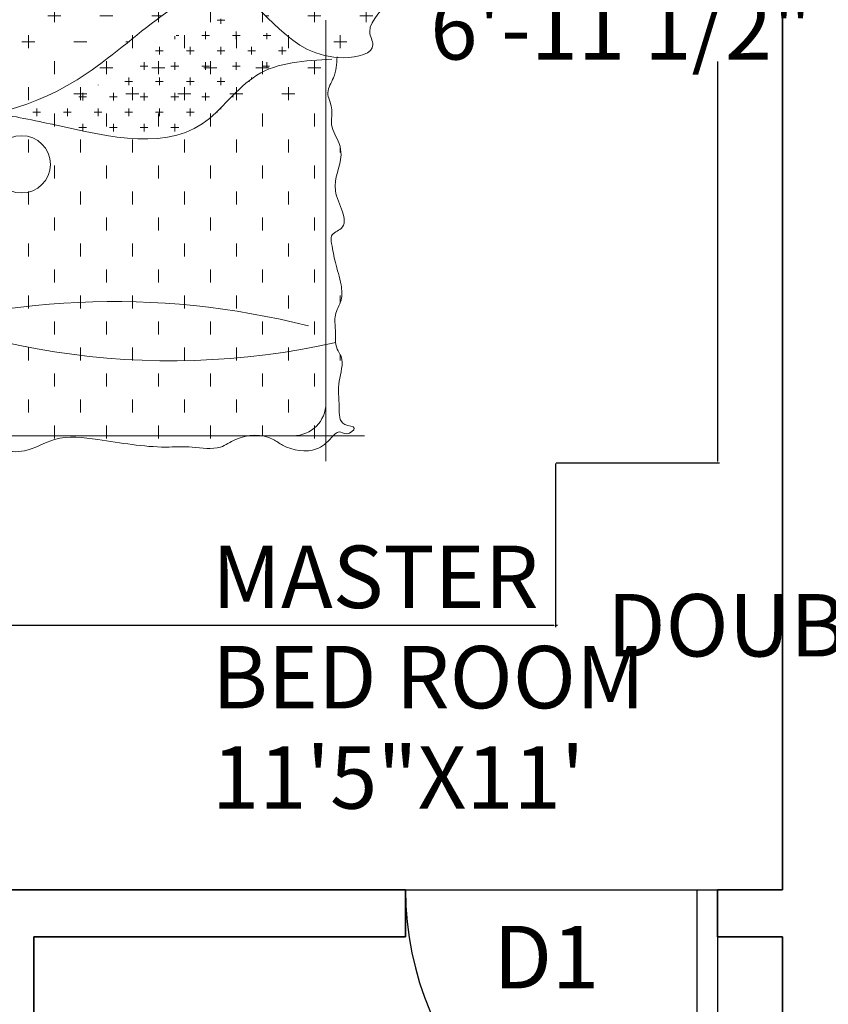
# Model space of a CAD drawing. Units: inches. Extents: x -26 to 575, y -18 to 513.
# Tile 12 of 28: x 196 to 274, y 324 to 418. Entities that reach past the tile are written whole.
import ezdxf

# ---------------------------------------------------------------- set-up
doc = ezdxf.new("R2010")
doc.units = ezdxf.units.IN
doc.header["$MEASUREMENT"] = 0
for name, color, linetype, lineweight in [('A-ANNO-DIMS', 2, 'Continuous', 18), ('A-ANNO-TEXT', 7, 'Continuous', 18), ('A-AREA-IDEN', 7, 'Continuous', 18), ('A-DOOR', 3, 'Continuous', 25), ('A-WALL', 7, 'Continuous', 35), ('Furniture', 8, 'Continuous', 15)]:
    doc.layers.add(name, color=color, linetype=linetype, lineweight=lineweight)
doc.styles.get("Standard").update_dxf_attribs({"font": 'arial.ttf', "height": 6})
doc.dimstyles.get("Standard").update_dxf_attribs({"dimtxt": 6, "dimasz": 0.18, "dimexe": 0.18, "dimexo": 0.0625, "dimgap": 0.09, "dimtad": 0, "dimtih": 1, "dimtoh": 1, "dimzin": 0, "dimdsep": 46, "dimlunit": 3, "dimtxsty": 'Standard', "dimcen": 0.09, "dimadec": 0, "dimazin": 0, "dimtfac": 1, "dimtofl": 0, "dimtmove": 0, "dimatfit": 3, "dimfxl": 1, "dimtolj": 1, "dimtzin": 0, "dimarcsym": 0})

# ---------------------------------------------------------------- blocks, each defined once
blk = doc.blocks.new('BED-DOUBLE-WITH-NIGHTSTANDS')
for p, q in [((1.925, 83.361), (1.925, 62.761)), ((82.669, 83.361), (82.669, 62.761)), ((21.61, 63.031), (21.61, 82.461)), ((22.828, 60.828), (22.828, 82.615)), ((81.883, 82.344), (81.883, 56.232)), ((102.354, 63.031), (102.354, 82.461)), ((10.269, 81.761), (8.938, 70.826)), ((23.226, 81.078), (0, 81.078)), ((21.24, 81.17), (81.883, 81.17)), ((103.97, 81.078), (80.744, 81.078)), ((20.889, 80.153), (2.667, 80.153)), ((2.667, 80.153), (2.667, 64.968)), ((20.889, 64.968), (20.889, 80.153)), ((82.669, 79.717), (21.062, 79.717)), ((101.633, 80.153), (83.411, 80.153)), ((83.411, 80.153), (83.411, 64.968)), ((101.633, 64.968), (101.633, 80.153)), ((92.567, 79.403), (92.567, 67.508)), ((14.667, 76.005), (4.51, 77.257)), ((25.057, 76.764), (22.828, 76.764)), ((41.168, 76.507), (40.96, 76.715)), ((41.168, 76.507), (41.434, 76.772)), ((41.169, 76.507), (41.169, 76.741)), ((56.226, 76.764), (41.357, 76.764)), ((43.997, 76.507), (43.732, 76.772)), ((43.997, 76.507), (43.997, 76.882)), ((43.997, 76.507), (44.262, 76.772)), ((46.825, 76.507), (46.56, 76.772)), ((46.825, 76.507), (47.09, 76.772)), ((46.826, 76.507), (46.826, 76.882)), ((57.003, 76.507), (56.737, 76.772)), ((57.003, 76.507), (57.003, 76.828)), ((57.003, 76.507), (57.268, 76.772)), ((81.883, 76.764), (59.394, 76.764)), ((59.831, 76.507), (59.594, 76.744)), ((59.831, 76.507), (59.831, 76.717)), ((59.831, 76.507), (60.018, 76.694)), ((8.056, 67.244), (12.026, 75.725)), ((12.026, 75.725), (14.235, 74.691)), ((11.458, 75.323), (8.122, 68.196)), ((11.769, 75.177), (11.458, 75.323)), ((25.612, 75.093), (25.347, 75.358)), ((25.612, 75.093), (25.612, 75.468)), ((25.612, 75.093), (25.877, 75.358)), ((28.44, 75.093), (28.175, 75.358)), ((28.44, 75.093), (28.706, 75.358)), ((28.441, 75.093), (28.441, 75.468)), ((31.269, 75.093), (31.004, 75.358)), ((31.269, 75.093), (31.269, 75.468)), ((31.269, 75.093), (31.534, 75.358)), ((34.097, 75.093), (33.832, 75.358)), ((34.097, 75.093), (34.362, 75.358)), ((34.098, 75.093), (34.098, 75.468)), ((36.926, 75.093), (36.661, 75.358)), ((36.926, 75.093), (36.926, 75.468)), ((36.926, 75.093), (37.191, 75.358)), ((39.754, 75.093), (39.489, 75.358)), ((39.754, 75.093), (40.019, 75.358)), ((39.755, 75.093), (39.755, 75.468)), ((42.583, 75.093), (42.317, 75.358)), ((42.583, 75.093), (42.583, 75.468)), ((42.583, 75.093), (42.848, 75.358)), ((45.411, 75.093), (45.146, 75.358)), ((45.411, 75.093), (45.411, 75.468)), ((45.411, 75.093), (45.676, 75.358)), ((48.239, 75.093), (47.974, 75.358)), ((48.239, 75.093), (48.505, 75.358)), ((48.24, 75.093), (48.24, 75.468)), ((51.068, 75.093), (50.803, 75.358)), ((51.068, 75.093), (51.068, 75.099)), ((51.068, 75.093), (51.07, 75.095)), ((53.004, 75.337), (53.025, 75.358)), ((55.588, 75.093), (55.323, 75.358)), ((55.588, 75.093), (55.854, 75.358)), ((55.589, 75.093), (55.589, 75.468)), ((58.417, 75.093), (58.152, 75.358)), ((58.417, 75.093), (58.417, 75.468)), ((58.417, 75.093), (58.682, 75.358)), ((61.245, 75.093), (60.98, 75.358)), ((61.245, 75.093), (61.51, 75.358)), ((61.246, 75.093), (61.246, 75.468)), ((64.074, 75.093), (63.809, 75.358)), ((64.074, 75.093), (64.074, 75.468)), ((64.074, 75.093), (64.339, 75.358)), ((66.902, 75.093), (66.637, 75.358)), ((66.902, 75.093), (67.167, 75.358)), ((66.903, 75.093), (66.903, 75.468)), ((69.731, 75.093), (69.465, 75.358)), ((69.731, 75.093), (69.731, 75.468)), ((69.731, 75.093), (69.996, 75.358)), ((72.559, 75.093), (72.294, 75.358)), ((72.559, 75.093), (72.559, 75.468)), ((72.559, 75.093), (72.824, 75.358)), ((75.387, 75.093), (75.122, 75.358)), ((75.387, 75.093), (75.653, 75.358)), ((75.388, 75.093), (75.388, 75.468)), ((78.216, 75.093), (77.951, 75.358)), ((78.216, 75.093), (78.216, 75.468)), ((78.216, 75.093), (78.481, 75.358)), ((14.235, 74.691), (10.265, 66.21)), ((19.14, 71.727), (13.978, 74.143)), ((27.026, 73.679), (26.761, 73.944)), ((27.026, 73.679), (27.291, 73.944)), ((27.027, 73.678), (27.027, 74.053)), ((29.855, 73.679), (29.589, 73.944)), ((29.855, 73.678), (29.855, 74.053)), ((29.855, 73.679), (30.12, 73.944)), ((32.683, 73.679), (32.418, 73.944)), ((32.683, 73.678), (32.683, 74.053)), ((32.683, 73.679), (32.948, 73.944)), ((35.512, 73.679), (35.246, 73.944)), ((35.512, 73.678), (35.512, 74.053)), ((35.512, 73.679), (35.777, 73.944)), ((38.34, 73.679), (38.075, 73.944)), ((38.34, 73.678), (38.34, 74.053)), ((38.34, 73.679), (38.605, 73.944)), ((41.168, 73.679), (40.903, 73.944)), ((41.168, 73.679), (41.434, 73.944)), ((41.169, 73.678), (41.169, 74.053)), ((43.997, 73.679), (43.732, 73.944)), ((43.997, 73.678), (43.997, 74.053)), ((43.997, 73.679), (44.262, 73.944)), ((46.825, 73.679), (46.56, 73.944)), ((46.825, 73.679), (47.09, 73.944)), ((46.826, 73.678), (46.826, 74.053)), ((49.654, 73.679), (49.388, 73.944)), ((49.654, 73.678), (49.654, 74.053)), ((49.654, 73.679), (49.919, 73.944)), ((54.174, 73.679), (53.909, 73.944)), ((54.174, 73.679), (54.439, 73.944)), ((54.175, 73.678), (54.175, 74.053)), ((57.003, 73.679), (56.737, 73.944)), ((57.003, 73.678), (57.003, 74.053)), ((57.003, 73.679), (57.268, 73.944)), ((59.831, 73.679), (59.566, 73.944)), ((59.831, 73.678), (59.831, 74.053)), ((59.831, 73.679), (60.096, 73.944)), ((62.66, 73.679), (62.394, 73.944)), ((62.66, 73.678), (62.66, 74.053)), ((62.66, 73.679), (62.925, 73.944)), ((65.488, 73.679), (65.223, 73.944)), ((65.488, 73.678), (65.488, 74.053)), ((65.488, 73.679), (65.753, 73.944)), ((68.316, 73.679), (68.051, 73.944)), ((68.316, 73.679), (68.582, 73.944)), ((68.317, 73.678), (68.317, 74.053)), ((71.145, 73.679), (70.88, 73.944)), ((71.145, 73.678), (71.145, 74.053)), ((71.145, 73.679), (71.41, 73.944)), ((73.973, 73.679), (73.708, 73.944)), ((73.973, 73.679), (74.238, 73.944)), ((73.974, 73.678), (73.974, 74.053)), ((76.802, 73.679), (76.536, 73.944)), ((76.802, 73.678), (76.802, 74.053)), ((76.802, 73.679), (77.067, 73.944)), ((79.63, 73.679), (79.365, 73.944)), ((79.63, 73.678), (79.63, 74.053)), ((79.63, 73.679), (79.895, 73.944)), ((13.242, 72.571), (11.033, 73.605)), ((14.129, 73), (11.598, 67.591)), ((17.984, 71.195), (14.129, 73)), ((98.466, 73.144), (86.668, 73.144)), ((25.612, 72.265), (25.347, 72.53)), ((25.612, 72.264), (25.612, 72.639)), ((25.612, 72.265), (25.877, 72.53)), ((28.44, 72.265), (28.175, 72.53)), ((28.44, 72.265), (28.706, 72.53)), ((28.441, 72.264), (28.441, 72.639)), ((31.269, 72.265), (31.004, 72.53)), ((31.269, 72.264), (31.269, 72.639)), ((31.269, 72.265), (31.534, 72.53)), ((34.097, 72.265), (33.832, 72.53)), ((34.097, 72.265), (34.362, 72.53)), ((34.098, 72.264), (34.098, 72.639)), ((36.926, 72.265), (36.661, 72.53)), ((36.926, 72.264), (36.926, 72.639)), ((36.926, 72.265), (37.191, 72.53)), ((39.754, 72.265), (39.489, 72.53)), ((39.754, 72.265), (40.019, 72.53)), ((39.755, 72.264), (39.755, 72.639)), ((42.583, 72.265), (42.317, 72.53)), ((42.583, 72.264), (42.583, 72.639)), ((42.583, 72.265), (42.848, 72.53)), ((45.411, 72.265), (45.146, 72.53)), ((45.411, 72.264), (45.411, 72.639)), ((45.411, 72.265), (45.676, 72.53)), ((48.239, 72.265), (47.974, 72.53)), ((48.239, 72.265), (48.505, 72.53)), ((48.24, 72.264), (48.24, 72.639)), ((55.588, 72.265), (55.323, 72.53)), ((55.588, 72.265), (55.854, 72.53)), ((55.589, 72.264), (55.589, 72.639)), ((58.417, 72.265), (58.152, 72.53)), ((58.417, 72.264), (58.417, 72.639)), ((58.417, 72.265), (58.682, 72.53)), ((61.245, 72.265), (60.98, 72.53)), ((61.245, 72.265), (61.51, 72.53)), ((61.246, 72.264), (61.246, 72.639)), ((64.074, 72.265), (63.809, 72.53)), ((64.074, 72.264), (64.074, 72.639)), ((64.074, 72.265), (64.339, 72.53)), ((66.902, 72.265), (66.637, 72.53)), ((66.902, 72.265), (67.167, 72.53)), ((66.903, 72.264), (66.903, 72.639)), ((69.731, 72.265), (69.465, 72.53)), ((69.731, 72.264), (69.731, 72.639)), ((69.731, 72.265), (69.996, 72.53)), ((72.559, 72.265), (72.294, 72.53)), ((72.559, 72.264), (72.559, 72.639)), ((72.559, 72.265), (72.824, 72.53)), ((75.387, 72.265), (75.122, 72.53)), ((75.387, 72.265), (75.653, 72.53)), ((75.388, 72.264), (75.388, 72.639)), ((78.216, 72.265), (77.951, 72.53)), ((78.216, 72.264), (78.216, 72.639)), ((78.216, 72.265), (78.481, 72.53)), ((15.452, 65.787), (17.984, 71.195)), ((15.804, 64.601), (19.14, 71.727)), ((24.198, 70.85), (23.972, 71.076)), ((24.198, 70.85), (24.198, 71.225)), ((24.198, 70.85), (24.463, 71.116)), ((27.026, 70.85), (26.761, 71.116)), ((27.026, 70.85), (27.291, 71.116)), ((27.027, 70.85), (27.027, 71.225)), ((29.855, 70.85), (29.589, 71.116)), ((29.855, 70.85), (29.855, 71.225)), ((29.855, 70.85), (30.12, 71.116)), ((32.683, 70.85), (32.418, 71.116)), ((32.683, 70.85), (32.683, 71.225)), ((32.683, 70.85), (32.948, 71.116)), ((35.512, 70.85), (35.246, 71.116)), ((35.512, 70.85), (35.512, 71.225)), ((35.512, 70.85), (35.777, 71.116)), ((38.34, 70.85), (38.075, 71.116)), ((38.34, 70.85), (38.34, 71.225)), ((38.34, 70.85), (38.605, 71.116)), ((41.168, 70.85), (40.903, 71.116)), ((41.168, 70.85), (41.434, 71.116)), ((41.169, 70.85), (41.169, 71.225)), ((43.997, 70.85), (43.732, 71.116)), ((43.997, 70.85), (43.997, 71.225)), ((43.997, 70.85), (44.262, 71.116)), ((46.825, 70.85), (46.56, 71.116)), ((46.825, 70.85), (47.09, 71.116)), ((46.826, 70.85), (46.826, 71.225)), ((49.654, 70.85), (49.388, 71.116)), ((49.654, 70.85), (49.654, 71.225)), ((49.654, 70.85), (49.919, 71.116)), ((54.174, 70.85), (53.909, 71.116)), ((54.174, 70.85), (54.439, 71.116)), ((54.175, 70.85), (54.175, 71.225)), ((57.003, 70.85), (56.737, 71.116)), ((57.003, 70.85), (57.003, 71.225)), ((57.003, 70.85), (57.268, 71.116)), ((59.831, 70.85), (59.566, 71.116)), ((59.831, 70.85), (59.831, 71.225)), ((59.831, 70.85), (60.096, 71.116)), ((62.66, 70.85), (62.394, 71.116)), ((62.66, 70.85), (62.66, 71.225)), ((62.66, 70.85), (62.925, 71.116)), ((65.488, 70.85), (65.223, 71.116)), ((65.488, 70.85), (65.488, 71.225)), ((65.488, 70.85), (65.753, 71.116)), ((68.316, 70.85), (68.051, 71.116)), ((68.316, 70.85), (68.582, 71.116)), ((68.317, 70.85), (68.317, 71.225)), ((71.145, 70.85), (70.88, 71.116)), ((71.145, 70.85), (71.145, 71.225)), ((71.145, 70.85), (71.41, 71.116)), ((73.973, 70.85), (73.708, 71.116)), ((73.973, 70.85), (74.238, 71.116)), ((73.974, 70.85), (73.974, 71.225)), ((76.802, 70.85), (76.536, 71.116)), ((76.802, 70.85), (76.802, 71.225)), ((76.802, 70.85), (77.067, 71.116)), ((79.63, 70.85), (79.365, 71.116)), ((79.63, 70.85), (79.63, 71.225)), ((79.63, 70.85), (79.895, 71.116)), ((11.136, 68.071), (8.927, 69.105)), ((25.612, 69.436), (25.347, 69.701)), ((25.612, 69.436), (25.612, 69.811)), ((25.612, 69.436), (25.877, 69.701)), ((28.44, 69.436), (28.175, 69.701)), ((28.44, 69.436), (28.706, 69.701)), ((28.441, 69.436), (28.441, 69.811)), ((31.269, 69.436), (31.004, 69.701)), ((31.269, 69.436), (31.269, 69.811)), ((31.269, 69.436), (31.534, 69.701)), ((34.097, 69.436), (33.832, 69.701)), ((34.097, 69.436), (34.362, 69.701)), ((34.098, 69.436), (34.098, 69.811)), ((36.926, 69.436), (36.661, 69.701)), ((36.926, 69.436), (36.926, 69.811)), ((36.926, 69.436), (37.191, 69.701)), ((39.754, 69.436), (39.489, 69.701)), ((39.754, 69.436), (40.019, 69.701)), ((39.755, 69.436), (39.755, 69.811)), ((42.583, 69.436), (42.317, 69.701)), ((42.583, 69.436), (42.583, 69.811)), ((42.583, 69.436), (42.848, 69.701)), ((45.411, 69.436), (45.146, 69.701)), ((45.411, 69.436), (45.411, 69.811)), ((45.411, 69.436), (45.676, 69.701)), ((48.239, 69.436), (47.974, 69.701)), ((48.239, 69.436), (48.505, 69.701)), ((48.24, 69.436), (48.24, 69.811)), ((51.052, 69.452), (50.803, 69.701)), ((53.007, 69.683), (53.025, 69.701)), ((55.588, 69.436), (55.323, 69.701)), ((55.588, 69.436), (55.854, 69.701)), ((55.589, 69.436), (55.589, 69.811)), ((58.417, 69.436), (58.152, 69.701)), ((58.417, 69.436), (58.417, 69.811)), ((58.417, 69.436), (58.682, 69.701)), ((61.245, 69.436), (60.98, 69.701)), ((61.245, 69.436), (61.51, 69.701)), ((61.246, 69.436), (61.246, 69.811)), ((64.074, 69.436), (63.809, 69.701)), ((64.074, 69.436), (64.074, 69.811)), ((64.074, 69.436), (64.339, 69.701)), ((66.902, 69.436), (66.637, 69.701)), ((66.902, 69.436), (67.167, 69.701)), ((66.903, 69.436), (66.903, 69.811)), ((69.731, 69.436), (69.465, 69.701)), ((69.731, 69.436), (69.731, 69.811)), ((69.731, 69.436), (69.996, 69.701)), ((72.559, 69.436), (72.294, 69.701)), ((72.559, 69.436), (72.559, 69.811)), ((72.559, 69.436), (72.824, 69.701)), ((75.387, 69.436), (75.122, 69.701)), ((75.387, 69.436), (75.653, 69.701)), ((75.388, 69.436), (75.388, 69.811)), ((78.216, 69.436), (77.951, 69.701)), ((78.216, 69.436), (78.216, 69.811)), ((78.216, 69.436), (78.481, 69.701)), ((8.122, 68.196), (8.434, 68.05)), ((24.198, 68.022), (23.933, 68.287)), ((24.198, 68.022), (24.198, 68.397)), ((24.198, 68.022), (24.463, 68.287)), ((27.026, 68.022), (26.761, 68.287)), ((27.026, 68.022), (27.291, 68.287)), ((27.027, 68.022), (27.027, 68.397)), ((29.855, 68.022), (29.589, 68.287)), ((29.855, 68.022), (29.855, 68.397)), ((29.855, 68.022), (30.12, 68.287)), ((32.683, 68.022), (32.418, 68.287)), ((32.683, 68.022), (32.683, 68.397)), ((32.683, 68.022), (32.948, 68.287)), ((35.512, 68.022), (35.246, 68.287)), ((35.512, 68.022), (35.512, 68.397)), ((35.512, 68.022), (35.777, 68.287)), ((38.34, 68.022), (38.075, 68.287)), ((38.34, 68.022), (38.34, 68.397)), ((38.34, 68.022), (38.605, 68.287)), ((41.168, 68.022), (40.903, 68.287)), ((41.168, 68.022), (41.434, 68.287)), ((41.169, 68.022), (41.169, 68.397)), ((43.997, 68.022), (43.732, 68.287)), ((43.997, 68.022), (43.997, 68.397)), ((43.997, 68.022), (44.262, 68.287)), ((46.825, 68.022), (46.56, 68.287)), ((46.825, 68.022), (47.09, 68.287)), ((46.826, 68.022), (46.826, 68.397)), ((49.654, 68.022), (49.388, 68.287)), ((49.654, 68.022), (49.654, 68.397)), ((49.654, 68.022), (49.919, 68.287)), ((54.174, 68.022), (53.909, 68.287)), ((54.174, 68.022), (54.439, 68.287)), ((54.175, 68.022), (54.175, 68.397)), ((57.003, 68.022), (56.737, 68.287)), ((57.003, 68.022), (57.003, 68.397)), ((57.003, 68.022), (57.268, 68.287)), ((59.831, 68.022), (59.566, 68.287)), ((59.831, 68.022), (59.831, 68.397)), ((59.831, 68.022), (60.096, 68.287)), ((62.66, 68.022), (62.394, 68.287)), ((62.66, 68.022), (62.66, 68.397)), ((62.66, 68.022), (62.925, 68.287)), ((65.488, 68.022), (65.223, 68.287)), ((65.488, 68.022), (65.488, 68.397)), ((65.488, 68.022), (65.753, 68.287)), ((68.316, 68.022), (68.051, 68.287)), ((68.316, 68.022), (68.582, 68.287)), ((68.317, 68.022), (68.317, 68.397)), ((71.145, 68.022), (70.88, 68.287)), ((71.145, 68.022), (71.145, 68.397)), ((71.145, 68.022), (71.41, 68.287)), ((73.973, 68.022), (73.708, 68.287)), ((73.973, 68.022), (74.238, 68.287)), ((73.974, 68.022), (73.974, 68.397)), ((76.802, 68.022), (76.536, 68.287)), ((76.802, 68.022), (76.802, 68.397)), ((76.802, 68.022), (77.067, 68.287)), ((79.63, 68.022), (79.365, 68.287)), ((79.63, 68.022), (79.63, 68.397)), ((79.63, 68.022), (79.895, 68.287)), ((10.265, 66.21), (8.056, 67.244)), ((11.598, 67.591), (15.452, 65.787)), ((10.642, 67.017), (15.804, 64.601)), ((25.612, 66.608), (25.347, 66.873)), ((25.612, 66.607), (25.612, 66.982)), ((25.612, 66.608), (25.877, 66.873)), ((28.44, 66.608), (28.175, 66.873)), ((28.44, 66.608), (28.706, 66.873)), ((28.441, 66.607), (28.441, 66.982)), ((31.269, 66.608), (31.004, 66.873)), ((31.269, 66.607), (31.269, 66.982)), ((31.269, 66.608), (31.534, 66.873)), ((34.097, 66.608), (33.832, 66.873)), ((34.097, 66.608), (34.362, 66.873)), ((34.098, 66.607), (34.098, 66.982)), ((36.926, 66.608), (36.661, 66.873)), ((36.926, 66.607), (36.926, 66.982)), ((36.926, 66.608), (37.191, 66.873)), ((39.754, 66.608), (39.489, 66.873)), ((39.754, 66.608), (40.019, 66.873)), ((39.755, 66.607), (39.755, 66.982)), ((42.583, 66.608), (42.317, 66.873)), ((42.583, 66.607), (42.583, 66.982)), ((42.583, 66.608), (42.848, 66.873)), ((45.411, 66.608), (45.146, 66.873)), ((45.411, 66.607), (45.411, 66.982)), ((45.411, 66.608), (45.676, 66.873)), ((48.239, 66.608), (47.974, 66.873)), ((48.239, 66.608), (48.505, 66.873)), ((48.24, 66.607), (48.24, 66.982)), ((51.068, 66.608), (50.803, 66.873)), ((51.068, 66.607), (51.068, 66.982)), ((51.068, 66.608), (51.333, 66.873)), ((52.76, 66.608), (52.495, 66.873)), ((52.76, 66.607), (52.76, 66.982)), ((52.76, 66.608), (53.025, 66.873)), ((55.588, 66.608), (55.323, 66.873)), ((55.588, 66.608), (55.854, 66.873)), ((55.589, 66.607), (55.589, 66.982)), ((58.417, 66.608), (58.152, 66.873)), ((58.417, 66.607), (58.417, 66.982)), ((58.417, 66.608), (58.682, 66.873)), ((61.245, 66.608), (60.98, 66.873)), ((61.245, 66.608), (61.51, 66.873)), ((61.246, 66.607), (61.246, 66.982)), ((64.074, 66.608), (63.809, 66.873)), ((64.074, 66.607), (64.074, 66.982)), ((64.074, 66.608), (64.339, 66.873)), ((66.902, 66.608), (66.637, 66.873)), ((66.902, 66.608), (67.167, 66.873)), ((66.903, 66.607), (66.903, 66.982)), ((69.731, 66.608), (69.465, 66.873)), ((69.731, 66.607), (69.731, 66.982)), ((69.731, 66.608), (69.996, 66.873)), ((72.559, 66.608), (72.294, 66.873)), ((72.559, 66.607), (72.559, 66.982)), ((72.559, 66.608), (72.824, 66.873)), ((75.387, 66.608), (75.122, 66.873)), ((75.387, 66.608), (75.653, 66.873)), ((75.388, 66.607), (75.388, 66.982)), ((78.216, 66.608), (77.951, 66.873)), ((78.216, 66.607), (78.216, 66.982)), ((78.216, 66.608), (78.481, 66.873)), ((81.044, 66.608), (80.779, 66.873)), ((81.044, 66.608), (81.253, 66.817)), ((81.045, 66.607), (81.045, 66.982)), ((24.198, 65.385), (24.198, 65.568)), ((24.295, 65.291), (24.463, 65.459)), ((27.026, 65.194), (26.761, 65.459)), ((27.026, 65.194), (27.291, 65.459)), ((27.027, 65.193), (27.027, 65.568)), ((29.855, 65.194), (29.589, 65.459)), ((29.855, 65.193), (29.855, 65.568)), ((29.855, 65.194), (30.12, 65.459)), ((32.683, 65.194), (32.418, 65.459)), ((32.683, 65.193), (32.683, 65.568)), ((32.683, 65.194), (32.948, 65.459)), ((35.335, 65.37), (35.246, 65.459)), ((35.512, 65.394), (35.512, 65.568)), ((35.743, 65.425), (35.777, 65.459)), ((46.774, 65.245), (46.56, 65.459)), ((46.826, 65.232), (46.826, 65.568)), ((46.856, 65.224), (47.09, 65.459)), ((49.654, 65.194), (49.388, 65.459)), ((49.654, 65.193), (49.654, 65.568)), ((49.654, 65.194), (49.919, 65.459)), ((54.174, 65.194), (53.909, 65.459)), ((54.174, 65.194), (54.439, 65.459)), ((54.175, 65.193), (54.175, 65.568)), ((57.003, 65.194), (56.737, 65.459)), ((57.003, 65.193), (57.003, 65.568)), ((57.003, 65.194), (57.268, 65.459)), ((59.831, 65.194), (59.566, 65.459)), ((59.831, 65.193), (59.831, 65.568)), ((59.831, 65.194), (60.096, 65.459)), ((62.66, 65.525), (62.66, 65.568)), ((65.488, 65.481), (65.488, 65.568)), ((65.74, 65.446), (65.753, 65.459)), ((68.316, 65.194), (68.051, 65.459)), ((68.316, 65.194), (68.582, 65.459)), ((68.317, 65.193), (68.317, 65.568)), ((71.145, 65.194), (70.88, 65.459)), ((71.145, 65.193), (71.145, 65.568)), ((71.145, 65.194), (71.41, 65.459)), ((73.973, 65.194), (73.708, 65.459)), ((73.973, 65.194), (74.238, 65.459)), ((73.974, 65.193), (73.974, 65.568)), ((76.802, 65.194), (76.536, 65.459)), ((76.802, 65.193), (76.802, 65.568)), ((76.802, 65.194), (77.067, 65.459)), ((79.63, 65.194), (79.365, 65.459)), ((79.63, 65.193), (79.63, 65.568)), ((79.63, 65.194), (79.895, 65.459)), ((82.154, 61.735), (82.154, 65.422)), ((2.667, 64.968), (20.889, 64.968)), ((83.411, 64.968), (101.633, 64.968)), ((0.451, 64.149), (23.136, 64.149)), ((55.589, 64.121), (55.589, 64.154)), ((81.194, 64.149), (103.88, 64.149)), ((78.267, 59.667), (78.267, 60.149)), ((20.767, 58.212), (20.767, 58.417)), ((21.392, 57.792), (21.312, 57.792)), ((26.392, 57.792), (25.142, 57.792)), ((25.767, 57.167), (25.767, 58.417)), ((31.392, 57.792), (30.142, 57.792)), ((30.767, 57.167), (30.767, 58.417)), ((36.392, 57.792), (35.142, 57.792)), ((35.767, 57.167), (35.767, 58.407)), ((41.392, 57.792), (40.142, 57.792)), ((40.767, 57.167), (40.767, 57.965)), ((60.767, 57.167), (60.767, 57.735)), ((66.392, 57.792), (65.142, 57.792)), ((65.767, 57.167), (65.767, 58.213)), ((71.392, 57.792), (70.142, 57.792)), ((70.767, 57.167), (70.767, 58.417)), ((76.392, 57.792), (75.142, 57.792)), ((75.767, 57.167), (75.767, 58.417)), ((81.392, 57.792), (80.142, 57.792)), ((80.767, 57.167), (80.767, 58.417)), ((45.767, 57.167), (45.767, 57.639)), ((50.767, 57.167), (50.767, 57.462)), ((55.767, 57.167), (55.767, 57.483)), ((28.267, 54.667), (28.267, 55.917)), ((33.267, 54.667), (33.267, 55.917)), ((38.267, 54.667), (38.267, 55.917)), ((43.267, 54.667), (43.267, 55.917)), ((48.267, 54.667), (48.267, 55.917)), ((53.267, 54.667), (53.267, 55.917)), ((58.267, 54.667), (58.267, 55.917)), ((63.267, 54.667), (63.267, 55.917)), ((68.267, 54.667), (68.267, 55.917)), ((73.267, 54.667), (73.267, 55.917)), ((78.267, 54.667), (78.267, 55.917)), ((83.267, 54.667), (83.267, 55.917)), ((23.273, 54.636), (23.273, 55.755)), ((28.892, 55.292), (27.642, 55.292)), ((33.892, 55.292), (32.642, 55.292)), ((38.892, 55.292), (37.642, 55.292)), ((43.892, 55.292), (42.642, 55.292)), ((48.892, 55.292), (47.642, 55.292)), ((53.892, 55.292), (52.642, 55.292)), ((58.892, 55.292), (57.642, 55.292)), ((63.892, 55.292), (62.642, 55.292)), ((68.892, 55.292), (67.642, 55.292)), ((73.892, 55.292), (72.642, 55.292)), ((78.892, 55.292), (77.642, 55.292)), ((83.892, 55.292), (82.642, 55.292)), ((30.767, 52.167), (30.767, 53.417)), ((35.767, 52.167), (35.767, 53.417)), ((40.767, 52.167), (40.767, 53.417)), ((45.767, 52.167), (45.767, 53.417)), ((50.767, 52.167), (50.767, 53.417)), ((55.767, 52.167), (55.767, 53.417)), ((60.767, 52.167), (60.767, 53.417)), ((65.767, 52.167), (65.767, 53.417)), ((70.767, 52.167), (70.767, 53.417)), ((75.767, 52.167), (75.767, 53.417)), ((80.767, 52.167), (80.767, 53.417)), ((26.392, 52.792), (25.619, 52.792)), ((31.392, 52.792), (30.142, 52.792)), ((36.392, 52.792), (35.142, 52.792)), ((41.392, 52.792), (40.142, 52.792)), ((46.392, 52.792), (45.142, 52.792)), ((51.392, 52.792), (50.142, 52.792)), ((56.392, 52.792), (55.142, 52.792)), ((61.392, 52.792), (60.142, 52.792)), ((66.392, 52.792), (65.142, 52.792)), ((71.392, 52.792), (70.142, 52.792)), ((76.392, 52.792), (75.142, 52.792)), ((81.392, 52.792), (80.142, 52.792)), ((23.892, 50.292), (22.642, 50.292)), ((23.267, 49.667), (23.267, 50.917)), ((28.892, 50.292), (27.642, 50.292)), ((28.267, 49.667), (28.267, 50.917)), ((33.892, 50.292), (32.642, 50.292)), ((33.267, 49.667), (33.267, 50.917)), ((38.892, 50.292), (37.642, 50.292)), ((38.267, 49.667), (38.267, 50.917)), ((43.892, 50.292), (42.642, 50.292)), ((43.267, 49.667), (43.267, 50.917)), ((48.892, 50.292), (47.642, 50.292)), ((48.267, 49.667), (48.267, 50.917)), ((53.892, 50.292), (52.642, 50.292)), ((53.267, 49.667), (53.267, 50.917)), ((58.892, 50.292), (57.642, 50.292)), ((58.267, 49.667), (58.267, 50.917)), ((63.892, 50.292), (62.642, 50.292)), ((63.267, 49.667), (63.267, 50.917)), ((68.892, 50.292), (67.642, 50.292)), ((68.267, 49.667), (68.267, 50.917)), ((73.892, 50.292), (72.642, 50.292)), ((73.267, 49.667), (73.267, 50.917)), ((78.892, 50.292), (77.642, 50.292)), ((78.267, 49.667), (78.267, 50.917)), ((83.892, 50.292), (82.642, 50.292)), ((83.267, 49.667), (83.267, 50.917)), ((20.767, 47.167), (20.767, 48.417)), ((30.767, 47.167), (30.767, 48.417)), ((35.767, 47.167), (35.767, 48.417)), ((40.767, 47.167), (40.767, 48.417)), ((45.767, 47.167), (45.767, 48.417)), ((50.767, 47.167), (50.767, 48.417)), ((55.767, 47.167), (55.767, 48.417)), ((65.767, 47.167), (65.767, 48.417)), ((70.767, 47.167), (70.767, 48.417)), ((75.767, 47.167), (75.767, 48.417)), ((80.767, 47.167), (80.767, 48.417)), ((21.392, 47.792), (20.412, 47.792)), ((26.392, 47.792), (25.142, 47.792)), ((31.392, 47.792), (30.142, 47.792)), ((36.392, 47.792), (35.142, 47.792)), ((41.392, 47.792), (40.142, 47.792)), ((46.392, 47.792), (45.142, 47.792)), ((51.392, 47.792), (50.142, 47.792)), ((56.392, 47.792), (55.142, 47.792)), ((66.392, 47.792), (65.142, 47.792)), ((71.392, 47.792), (70.142, 47.792)), ((76.392, 47.792), (75.142, 47.792)), ((81.392, 47.792), (80.142, 47.792)), ((23.267, 44.667), (23.267, 45.917)), ((28.267, 44.667), (28.267, 45.917)), ((33.267, 44.667), (33.267, 45.917)), ((38.267, 44.667), (38.267, 45.917)), ((43.267, 44.667), (43.267, 45.917)), ((48.267, 44.667), (48.267, 45.917)), ((53.267, 44.667), (53.267, 45.917)), ((63.267, 44.667), (63.267, 45.917)), ((68.267, 44.667), (68.267, 45.917)), ((73.267, 44.667), (73.267, 45.917)), ((78.267, 44.667), (78.267, 45.917)), ((83.267, 44.667), (83.267, 45.917)), ((23.892, 45.292), (22.642, 45.292)), ((28.892, 45.292), (27.642, 45.292)), ((33.892, 45.292), (32.642, 45.292)), ((38.892, 45.292), (37.642, 45.292)), ((43.892, 45.292), (42.642, 45.292)), ((48.892, 45.292), (47.642, 45.292)), ((53.892, 45.292), (52.642, 45.292)), ((58.892, 45.292), (57.642, 45.292)), ((63.892, 45.292), (62.642, 45.292)), ((68.892, 45.292), (67.642, 45.292)), ((73.892, 45.292), (72.642, 45.292)), ((78.892, 45.292), (77.642, 45.292)), ((83.892, 45.292), (82.642, 45.292)), ((21.392, 42.792), (20.142, 42.792)), ((20.767, 42.167), (20.767, 43.417)), ((26.392, 42.792), (25.142, 42.792)), ((31.392, 42.792), (30.142, 42.792)), ((30.767, 42.167), (30.767, 43.417)), ((36.392, 42.792), (35.142, 42.792)), ((35.767, 42.167), (35.767, 43.417)), ((41.392, 42.792), (40.142, 42.792)), ((40.767, 42.167), (40.767, 43.417)), ((46.392, 42.792), (45.142, 42.792)), ((45.767, 42.167), (45.767, 43.417)), ((51.392, 42.792), (50.142, 42.792)), ((50.767, 42.167), (50.767, 43.417)), ((56.392, 42.792), (55.142, 42.792)), ((55.767, 42.167), (55.767, 43.417)), ((61.392, 42.792), (60.142, 42.792)), ((66.089, 42.792), (65.142, 42.792)), ((65.767, 42.167), (65.767, 43.417)), ((70.767, 42.167), (70.767, 43.417)), ((75.767, 42.167), (75.767, 43.417)), ((76.392, 42.792), (76.07, 42.792)), ((81.392, 42.792), (80.142, 42.792)), ((80.767, 42.167), (80.767, 43.417)), ((86.392, 42.792), (85.142, 42.792)), ((85.767, 42.167), (85.767, 43.417)), ((72.149, 42.386), (71.41, 42.386)), ((71.779, 42.017), (71.779, 42.495)), ((81.883, 42.36), (81.883, 0)), ((18.267, 39.667), (18.267, 40.917)), ((23.267, 39.991), (23.267, 40.917)), ((28.267, 39.667), (28.267, 40.917)), ((33.267, 39.667), (33.267, 40.917)), ((38.267, 39.667), (38.267, 40.917)), ((43.267, 39.667), (43.267, 40.917)), ((48.267, 39.667), (48.267, 40.917)), ((53.267, 39.667), (53.267, 40.917)), ((63.267, 39.667), (63.267, 40.917)), ((67.35, 40.541), (67.35, 40.835)), ((67.719, 40.91), (67.48, 40.91)), ((68.267, 39.667), (68.267, 40.917)), ((70.672, 40.91), (69.934, 40.91)), ((70.303, 40.541), (70.303, 41.279)), ((73.625, 40.91), (72.887, 40.91)), ((73.256, 40.541), (73.256, 41.279)), ((73.267, 39.667), (73.267, 40.917)), ((76.578, 40.91), (75.839, 40.91)), ((76.209, 40.541), (76.209, 41.133)), ((78.267, 39.667), (78.267, 40.917)), ((83.267, 39.667), (83.267, 40.917)), ((18.892, 40.292), (17.831, 40.292)), ((23.892, 40.292), (22.642, 40.292)), ((28.892, 40.292), (27.642, 40.292)), ((33.892, 40.292), (32.642, 40.292)), ((38.892, 40.292), (37.642, 40.292)), ((43.892, 40.292), (42.642, 40.292)), ((48.892, 40.292), (47.642, 40.292)), ((53.892, 40.292), (52.642, 40.292)), ((58.892, 40.292), (57.642, 40.292)), ((62.901, 40.292), (62.642, 40.292)), ((65.874, 39.064), (65.874, 39.802)), ((68.827, 39.064), (68.827, 39.802)), ((71.779, 39.064), (71.779, 39.802)), ((74.732, 39.064), (74.732, 39.802)), ((77.685, 39.064), (77.685, 39.802)), ((83.892, 40.292), (82.642, 40.292)), ((22.828, 3.418), (22.828, 38.865)), ((66.243, 39.433), (65.505, 39.433)), ((69.196, 39.433), (68.458, 39.433)), ((72.149, 39.433), (71.41, 39.433)), ((75.101, 39.433), (74.363, 39.433)), ((78.054, 39.433), (77.316, 39.433)), ((25.767, 37.167), (25.767, 38.417)), ((30.767, 37.167), (30.767, 38.417)), ((35.767, 37.167), (35.767, 38.417)), ((40.767, 37.167), (40.767, 38.417)), ((45.767, 37.167), (45.767, 38.417)), ((50.767, 37.167), (50.767, 38.417)), ((55.767, 37.167), (55.767, 38.417)), ((60.767, 37.167), (60.767, 38.417)), ((64.767, 37.957), (64.028, 37.957)), ((64.398, 37.588), (64.398, 38.326)), ((65.767, 37.167), (65.767, 38.417)), ((67.719, 37.957), (66.981, 37.957)), ((67.35, 37.588), (67.35, 38.326)), ((70.672, 37.957), (69.934, 37.957)), ((70.303, 37.588), (70.303, 38.326)), ((70.767, 37.167), (70.767, 38.417)), ((73.625, 37.957), (72.887, 37.957)), ((73.256, 37.588), (73.256, 38.326)), ((75.767, 37.167), (75.767, 38.417)), ((76.451, 37.957), (75.839, 37.957)), ((76.209, 37.798), (76.209, 38.326)), ((80.767, 37.167), (80.767, 38.417)), ((61.392, 37.792), (60.142, 37.792)), ((66.392, 37.792), (65.142, 37.792)), ((71.392, 37.792), (70.142, 37.792)), ((76.392, 37.792), (75.142, 37.792)), ((81.392, 37.792), (80.142, 37.792)), ((59.968, 36.111), (59.968, 36.158)), ((63.29, 36.481), (62.552, 36.481)), ((62.921, 36.111), (62.921, 36.85)), ((66.243, 36.481), (65.505, 36.481)), ((65.874, 36.111), (65.874, 36.85)), ((69.196, 36.481), (68.458, 36.481)), ((68.827, 36.111), (68.827, 36.85)), ((72.149, 36.481), (71.41, 36.481)), ((71.779, 36.111), (71.779, 36.85)), ((74.53, 36.481), (74.363, 36.481)), ((74.732, 36.661), (74.732, 36.85)), ((17.658, 35.292), (17.642, 35.292)), ((28.267, 34.667), (28.267, 35.917)), ((33.267, 34.667), (33.267, 35.917)), ((38.267, 34.667), (38.267, 35.917)), ((43.267, 34.667), (43.267, 35.917)), ((48.267, 34.667), (48.267, 35.917)), ((53.267, 34.667), (53.267, 35.917)), ((58.892, 35.292), (57.642, 35.292)), ((58.267, 34.667), (58.267, 35.917)), ((58.492, 34.635), (58.492, 35.373)), ((61.445, 34.635), (61.445, 35.373)), ((63.892, 35.292), (62.642, 35.292)), ((63.267, 34.667), (63.267, 35.917)), ((64.398, 34.635), (64.398, 35.373)), ((67.35, 34.635), (67.35, 35.373)), ((68.892, 35.292), (67.642, 35.292)), ((68.267, 34.667), (68.267, 35.917)), ((70.303, 34.635), (70.303, 35.373)), ((73.892, 35.292), (72.642, 35.292)), ((73.256, 35.252), (73.256, 35.373)), ((73.267, 34.667), (73.267, 35.917)), ((78.892, 35.292), (77.642, 35.292)), ((78.267, 34.667), (78.267, 35.917)), ((58.861, 35.004), (58.123, 35.004)), ((61.814, 35.004), (61.076, 35.004)), ((64.767, 35.004), (64.028, 35.004)), ((67.719, 35.004), (66.981, 35.004)), ((70.672, 35.004), (69.934, 35.004)), ((73.008, 35.004), (72.887, 35.004)), ((25.767, 32.167), (25.767, 33.417)), ((30.767, 32.167), (30.767, 33.417)), ((35.767, 32.167), (35.767, 33.417)), ((40.767, 32.167), (40.767, 33.417)), ((45.767, 32.167), (45.767, 33.417)), ((50.767, 32.167), (50.767, 33.417)), ((51.11, 33.245), (51.11, 33.484)), ((54.432, 33.528), (53.694, 33.528)), ((54.063, 33.159), (54.063, 33.897)), ((55.767, 32.167), (55.767, 33.417)), ((57.385, 33.528), (56.647, 33.528)), ((57.016, 33.159), (57.016, 33.897)), ((60.338, 33.528), (59.599, 33.528)), ((59.968, 33.159), (59.968, 33.897)), ((60.767, 32.167), (60.767, 33.417)), ((63.29, 33.528), (62.552, 33.528)), ((62.921, 33.159), (62.921, 33.897)), ((66.243, 33.528), (65.505, 33.528)), ((65.767, 32.167), (65.767, 33.417)), ((65.874, 33.159), (65.874, 33.897)), ((69.196, 33.528), (68.458, 33.528)), ((68.827, 33.159), (68.827, 33.897)), ((70.767, 32.167), (70.767, 33.417)), ((71.469, 33.528), (71.41, 33.528)), ((71.779, 33.808), (71.779, 33.897)), ((75.767, 32.167), (75.767, 33.417)), ((80.767, 32.167), (80.767, 33.417)), ((55.539, 32.371), (55.539, 32.421)), ((58.492, 31.744), (58.492, 32.421)), ((61.445, 31.682), (61.445, 32.421)), ((64.398, 31.682), (64.398, 32.421)), ((67.35, 31.682), (67.35, 32.421)), ((58.861, 32.051), (58.123, 32.051)), ((61.814, 32.051), (61.076, 32.051)), ((64.767, 32.051), (64.028, 32.051)), ((67.719, 32.051), (66.981, 32.051)), ((28.267, 29.667), (28.267, 30.917)), ((33.267, 29.667), (33.267, 30.917)), ((38.267, 29.667), (38.267, 30.917)), ((43.267, 29.667), (43.267, 30.917)), ((48.267, 29.667), (48.267, 30.917)), ((53.267, 29.667), (53.267, 30.917)), ((58.267, 29.667), (58.267, 30.917)), ((63.267, 29.667), (63.267, 30.917)), ((68.267, 29.667), (68.267, 30.917)), ((73.267, 29.667), (73.267, 30.917)), ((78.267, 29.667), (78.267, 30.917)), ((83.267, 29.667), (83.267, 30.107)), ((25.767, 27.167), (25.767, 28.417)), ((30.767, 27.167), (30.767, 28.417)), ((35.767, 27.167), (35.767, 28.417)), ((40.767, 27.167), (40.767, 28.417)), ((45.767, 27.167), (45.767, 28.417)), ((50.767, 27.167), (50.767, 28.417)), ((55.767, 27.167), (55.767, 28.417)), ((60.767, 27.167), (60.767, 28.417)), ((65.767, 27.167), (65.767, 28.417)), ((70.767, 27.167), (70.767, 28.417)), ((75.767, 27.167), (75.767, 28.417)), ((80.767, 27.167), (80.767, 28.417)), ((28.267, 24.667), (28.267, 25.917)), ((33.267, 24.667), (33.267, 25.917)), ((38.267, 24.667), (38.267, 25.917)), ((43.267, 24.667), (43.267, 25.917)), ((48.267, 24.667), (48.267, 25.917)), ((53.267, 24.667), (53.267, 25.917)), ((58.267, 24.667), (58.267, 25.917)), ((63.267, 24.667), (63.267, 25.917)), ((68.267, 24.667), (68.267, 25.917)), ((73.267, 24.667), (73.267, 25.917)), ((78.267, 24.667), (78.267, 25.917)), ((25.767, 22.167), (25.767, 23.417)), ((30.767, 22.167), (30.767, 23.417)), ((35.767, 22.167), (35.767, 23.417)), ((40.767, 22.167), (40.767, 23.417)), ((45.767, 22.167), (45.767, 23.417)), ((50.767, 22.167), (50.767, 23.417)), ((55.767, 22.167), (55.767, 23.417)), ((60.767, 22.167), (60.767, 23.417)), ((65.767, 22.167), (65.767, 23.417)), ((70.767, 22.167), (70.767, 23.417)), ((75.767, 22.167), (75.767, 23.417)), ((80.767, 22.167), (80.767, 23.417)), ((28.267, 19.667), (28.267, 20.917)), ((33.267, 19.667), (33.267, 20.917)), ((38.267, 19.667), (38.267, 20.917)), ((43.267, 19.667), (43.267, 20.917)), ((48.267, 19.667), (48.267, 20.917)), ((53.267, 19.667), (53.267, 20.917)), ((58.267, 19.667), (58.267, 20.917)), ((63.267, 19.667), (63.267, 20.917)), ((68.267, 19.667), (68.267, 20.917)), ((73.267, 19.667), (73.267, 20.917)), ((78.267, 19.667), (78.267, 20.917)), ((25.767, 17.168), (25.767, 18.417)), ((30.767, 17.168), (30.767, 18.417)), ((35.767, 17.168), (35.767, 18.417)), ((40.767, 17.168), (40.767, 18.417)), ((45.767, 17.168), (45.767, 18.417)), ((50.767, 17.168), (50.767, 18.417)), ((55.767, 17.168), (55.767, 18.417)), ((60.767, 17.168), (60.767, 18.417)), ((65.767, 17.168), (65.767, 18.417)), ((70.767, 17.168), (70.767, 18.417)), ((75.767, 17.168), (75.767, 18.417)), ((80.767, 17.168), (80.767, 18.417)), ((28.267, 14.668), (28.267, 15.918)), ((33.267, 14.668), (33.267, 15.918)), ((38.267, 14.668), (38.267, 15.918)), ((43.267, 14.668), (43.267, 15.918)), ((48.267, 14.668), (48.267, 15.918)), ((53.267, 14.668), (53.267, 15.918)), ((58.267, 14.668), (58.267, 15.918)), ((63.267, 14.668), (63.267, 15.918)), ((68.267, 14.668), (68.267, 15.918)), ((73.267, 14.668), (73.267, 15.918)), ((78.267, 14.668), (78.267, 15.918)), ((83.267, 15.255), (83.267, 15.918)), ((25.767, 12.168), (25.767, 13.418)), ((30.767, 12.168), (30.767, 13.418)), ((35.767, 12.168), (35.767, 13.418)), ((40.767, 12.168), (40.767, 13.418)), ((45.767, 12.168), (45.767, 13.418)), ((50.767, 12.168), (50.767, 13.418)), ((55.767, 12.168), (55.767, 13.418)), ((60.767, 12.168), (60.767, 13.418)), ((65.767, 12.168), (65.767, 13.418)), ((70.767, 12.168), (70.767, 13.418)), ((75.767, 12.168), (75.767, 13.418)), ((80.767, 12.168), (80.767, 13.418)), ((28.267, 9.668), (28.267, 10.918)), ((33.267, 9.668), (33.267, 10.918)), ((38.267, 9.668), (38.267, 10.918)), ((43.267, 9.668), (43.267, 10.918)), ((48.267, 9.668), (48.267, 10.918)), ((53.267, 9.668), (53.267, 10.918)), ((58.267, 9.668), (58.267, 10.918)), ((63.267, 9.668), (63.267, 10.918)), ((68.267, 9.668), (68.267, 10.918)), ((73.267, 9.668), (73.267, 10.918)), ((78.267, 9.668), (78.267, 10.918)), ((83.267, 9.668), (83.267, 10.196)), ((22.115, 7.867), (21.706, 7.867)), ((25.767, 7.168), (25.767, 8.418)), ((30.767, 7.168), (30.767, 8.418)), ((35.767, 7.168), (35.767, 8.418)), ((40.767, 7.168), (40.767, 8.418)), ((45.767, 7.168), (45.767, 8.418)), ((50.767, 7.168), (50.767, 8.418)), ((55.767, 7.168), (55.767, 8.418)), ((60.767, 7.168), (60.767, 8.418)), ((65.767, 7.168), (65.767, 8.418)), ((70.767, 7.168), (70.767, 8.418)), ((75.767, 7.168), (75.767, 8.418)), ((80.767, 7.168), (80.767, 8.418)), ((28.267, 4.668), (28.267, 5.918)), ((33.267, 4.668), (33.267, 5.918)), ((38.267, 4.668), (38.267, 5.918)), ((43.267, 4.668), (43.267, 5.918)), ((48.267, 4.668), (48.267, 5.918)), ((53.267, 4.668), (53.267, 5.918)), ((58.267, 4.668), (58.267, 5.918)), ((63.267, 4.668), (63.267, 5.918)), ((68.267, 4.668), (68.267, 5.918)), ((73.267, 4.668), (73.267, 5.918)), ((78.267, 4.668), (78.267, 5.918)), ((25.767, 2.168), (25.767, 3.418)), ((30.767, 2.465), (30.767, 3.418)), ((35.767, 3.004), (35.767, 3.418)), ((40.767, 2.745), (40.767, 3.418)), ((45.767, 2.168), (45.767, 3.418)), ((50.767, 2.168), (50.767, 3.418)), ((55.767, 2.168), (55.767, 3.418)), ((60.767, 2.168), (60.767, 3.418)), ((65.767, 2.168), (65.767, 3.418)), ((70.767, 2.168), (70.767, 3.418)), ((75.767, 2.413), (75.767, 3.418)), ((80.767, 2.168), (80.767, 3.418)), ((85.58, 2.43), (23.697, 2.43)), ((36.392, 2.793), (35.142, 2.793)), ((40.395, 2.793), (40.142, 2.793))]:
    blk.add_line(p, q)
for centre, radius in [((9.65, 76.677), 4.065), ((9.65, 76.677), 3.73), ((9.65, 76.677), 1.87), ((9.65, 76.677), 1.702), ((92.824, 73.144), 3.847), ((92.824, 73.144), 2.272), ((60.492, 47.373), 2.359), ((52.627, 28.516), 2.753)]:
    blk.add_circle(centre, radius)
for centre, radius, start, end in [((40.615, 70.411), 11.457, 327.75554, 34.13971), ((18.641, 72.674), 7.534, 354.32477, 27.77276), ((41.09, 50.385), 26.004, 95.02643, 117.32994), ((64.238, 66.161), 9.788, 78.78839, 122.5362), ((83.338, 72.35), 4.658, 124.73446, 186.55264), ((44.415, 57.102), 10.589, 48.87132, 93.34478), ((76.199, 84.696), 20.356, 248.18569, 275.91055), ((27.055, 44.467), 7.557, 311.04012, 36.13845), ((86.259, 43.416), 4.944, 128.83543, 178.00379), ((39.784, 19.641), 17.214, 170.06779, 270.93205), ((30.825, 21.414), 8.013, 183.53609, 317.84857), ((66.971, 82.605), 72.965, 239.8126, 282.54723), ((41.047, 10.13), 8.244, 134.23532, 249.05847), ((61.483, -60.526), 75.853, 75.71433, 109.44594), ((25.975, 5.579), 3.15, 180, 270), ((78.733, 5.579), 3.15, 270, 0)]:
    blk.add_arc(centre, radius, start, end)
for points, knots in [([(24.713, 64.661), (26.06, 64.632), (33.003, 64.48), (41.955, 67.204), (49.025, 64.485), (52.786, 64.865), (50.633, 69.88), (50.431, 72.758), (51.756, 76.03), (43.447, 78.051), (36.588, 75.072), (28.311, 76.389), (25.374, 76.358), (24.839, 76.353)], [0, 0, 0, 0, 4.049674, 20.880819, 25.932041, 26.821979, 31.217024, 36.043065, 37.533831, 40.150607, 55.448466, 62.672935, 64.278467, 64.278467, 64.278467, 64.278467]), ([(81.301, 78.042), (80.682, 75.308), (79.671, 70.849), (81.18, 67.616), (83.379, 62.518), (82.094, 64.567), (81.589, 64.661)], [0, 0, 0, 0, 7.603099, 12.404488, 14.892294, 16.432626, 16.432626, 16.432626, 16.432626]), ([(25.073, 76.86), (24.732, 74.842), (24.154, 71.41), (22.763, 66.411), (24.846, 64.896), (25.601, 63.748), (26.066, 63.834)], [0, 0, 0, 0, 6.47304, 11.006869, 12.799679, 14.2185, 14.2185, 14.2185, 14.2185]), ([(81.33, 64.661), (77.466, 64.343), (71.206, 63.827), (62.265, 66.782), (55.978, 62.892), (52.048, 65.922), (52.93, 69.57), (53.856, 72.566), (52.444, 75.929), (58.704, 77.688), (63.648, 75.449), (70.131, 76.236), (74.451, 76.625), (78.12, 76.323), (80.316, 76.345), (81.042, 76.353)], [0, 0, 0, 0, 11.502554, 18.635017, 27.654655, 28.800011, 32.595859, 36.914018, 38.927328, 41.544104, 52.009639, 56.262652, 60.661637, 65.075538, 67.252844, 67.252844, 67.252844, 67.252844]), ([(81.883, 65.422), (81.768, 63.582), (81.624, 61.268), (84.254, 59.709), (83.774, 58.738), (83.516, 58.215)], [0, 0, 0, 0, 4.973031, 6.254082, 7.747585, 7.747585, 7.747585, 7.747585]), ([(83.91, 58.069), (84.557, 56.735), (85.575, 54.637), (82.278, 53.65), (82.991, 50.721), (85.334, 50.529), (84.903, 48.234), (82.063, 47.247), (85.774, 45.875), (88.761, 44.174), (85.372, 42.034), (87.053, 39.3), (78.856, 37.339), (72.977, 51.01), (54.082, 29.239), (35.907, 32.924), (20.82, 41.987), (17.166, 32.566), (16.239, 37.799), (18.713, 38.787), (15.912, 43.442), (22.37, 43.447), (20.934, 46.182), (20.192, 47.949), (20.317, 52.932), (35.125, 52.602), (16.252, 58.944), (26.308, 59.478), (35.165, 58.384), (54.321, 56.67), (69.444, 58.458), (82.072, 60.876), (83.528, 58.651), (83.91, 58.069)], [0, 0, 0, 0, 3.481099, 5.475811, 8.043407, 9.436812, 11.330727, 12.888379, 16.258255, 18.252967, 21.734596, 23.018392, 26.087149, 38.445812, 54.5649, 86.600283, 92.594507, 98.286547, 100.905288, 101.70342, 105.471876, 109.954916, 110.954151, 113.598333, 116.114301, 124.231953, 133.25029, 137.509046, 143.991555, 164.906349, 189.961005, 195.579007, 197.573325, 197.573325, 197.573325, 197.573325]), ([(23.431, 55.191), (24.486, 55.003), (27.111, 54.537), (29.416, 53.175), (30.793, 52.361)], [0, 0, 0, 0, 3.194191, 7.94245, 7.94245, 7.94245, 7.94245]), ([(83.725, 54.2), (82.764, 53.378), (78.971, 50.136), (73.792, 50.033), (69.926, 49.956)], [0, 0, 0, 0, 3.737027, 14.742384, 14.742384, 14.742384, 14.742384]), ([(82.947, 38.85), (82.911, 38.17), (82.846, 36.973), (81.755, 35.426), (82.665, 33.92), (82.165, 32.163), (83.168, 30.812), (83.54, 28.604), (81.842, 26.134), (84.594, 22.622), (82.267, 21.856), (82.5, 20.483), (82.772, 18.979), (83.36, 17.209), (83.496, 15.407), (82.607, 14.088), (82.874, 12.456), (82.705, 11.038), (83.722, 9.614), (82.912, 7.552), (83.231, 5.577), (83.079, 3.385), (85.076, 3.343), (83.878, 2.357), (83.088, 3.036), (82.19, 1.93), (80.715, 0.693), (78.274, 1.051), (76.159, 2.631), (73.682, 2.579), (71.479, 0.955), (69.048, 1.473), (65.151, 1.192), (60.806, 1.999), (56.053, 2.59), (52.446, 0.271), (49.194, 1.511), (46.115, 1.703), (37.688, 3.671), (31.84, 3.182), (20.439, -0.093), (22.209, 3.754), (19.175, -0.438), (22.913, 0.393), (27.139, 0.628), (21.628, 1.854), (19.679, 4.269), (19.873, 11.16), (24.262, 3.836), (20.295, 10.756), (23.261, 12.851), (24.334, 17.429), (16.78, 17.59), (25.964, 19.233), (16.198, 20.678), (24.666, 22.01), (20.037, 24.956), (24.596, 28.15), (20.032, 29.602), (23.483, 31.603), (22.431, 34.552), (22.916, 41.177), (22.854, 37.063), (22.828, 35.348)], [0, 0, 0, 0, 2.033881, 3.581387, 5.07489, 6.704853, 8.655612, 9.757262, 13.24098, 16.903694, 18.063816, 18.788243, 20.635227, 22.875483, 24.324336, 25.871843, 27.320698, 29.140811, 29.950855, 32.312207, 34.847704, 36.565952, 37.541804, 38.447727, 39.194923, 40.100844, 41.912688, 45.194843, 46.251388, 49.875946, 51.496686, 54.215105, 56.7523, 63.316606, 67.484853, 70.581422, 75.324573, 76.965649, 79.915763, 100.671038, 102.483321, 104.317501, 106.523635, 109.038061, 111.571263, 115.809372, 117.667229, 122.411431, 125.445794, 129.976907, 132.758854, 136.424739, 139.918708, 143.481583, 147.135325, 151.002466, 153.252794, 157.23352, 159.244583, 161.905351, 164.097269, 169.015093, 172.531686, 172.531686, 172.531686, 172.531686]), ([(82.451, 38.629), (79.861, 38.486), (74.81, 38.206), (68.702, 28.856), (57.628, 32.104), (43.09, 34.698), (32.134, 32.977), (18.889, 30.822), (17.485, 34.151), (16.98, 35.349)], [0, 0, 0, 0, 7.385187, 14.402621, 29.694422, 35.583277, 59.348121, 65.733553, 69.320983, 69.320983, 69.320983, 69.320983])]:
    blk.add_open_spline(points, degree=3, knots=knots)
blk = doc.blocks.new('DOOR-SWING-30IN')
for p, q in [((-30, 0), (0, 0)), ((-2, 0), (-2, -30)), ((0, 0), (0, -30))]:
    blk.add_line(p, q)
blk.add_arc((0, 0), 30, 180, 270)
blk = doc.blocks.new('*D12')
at = {"layer": 'A-ANNO-DIMS', "color": 0, "lineweight": -2, "transparency": 16777216}
for p, q in [((143.378, 375.468), (143.378, 359.755)), ((247.348, 375.468), (247.348, 359.755)), ((143.558, 359.935), (247.168, 359.935)), ((247.348, 359.935), (247.528, 359.935))]:
    blk.add_line(p, q, dxfattribs=at)
at = {"layer": 'A-ANNO-DIMS', "color": 0, "transparency": 16777216}
for points in [[(143.558, 359.965), (143.558, 359.905), (143.378, 359.935)], [(247.168, 359.965), (247.168, 359.905), (247.348, 359.935)]]:
    blk.add_solid(points, dxfattribs=at)
at = {"layer": 'Defpoints', "color": 0, "transparency": 16777216}
for p in [(143.378, 375.531), (247.348, 375.531), (247.348, 359.935)]:
    blk.add_point(p, dxfattribs=at)
at = {"layer": 'A-ANNO-DIMS', "color": 0, "transparency": 16777216, "insert": (329.097, 359.935), "char_height": 6, "attachment_point": 5}
blk.add_mtext('\\A1;DOUBLE BED & NIGHTSTANDS 8\'-8" TYP.', dxfattribs=at)
blk = doc.blocks.new('*D13')
at = {"layer": 'A-ANNO-DIMS', "color": 0, "lineweight": -2, "transparency": 16777216}
for p, q in [((247.41, 459.077), (263.123, 459.077)), ((262.943, 458.897), (262.943, 420.496)), ((262.943, 375.711), (262.943, 414.111)), ((247.41, 375.531), (263.123, 375.531))]:
    blk.add_line(p, q, dxfattribs=at)
at = {"layer": 'A-ANNO-DIMS', "color": 0, "transparency": 16777216}
for points in [[(262.913, 458.897), (262.973, 458.897), (262.943, 459.077)], [(262.913, 375.711), (262.973, 375.711), (262.943, 375.531)]]:
    blk.add_solid(points, dxfattribs=at)
at = {"layer": 'Defpoints', "color": 0, "transparency": 16777216}
for p in [(247.348, 459.077), (262.943, 459.077), (247.348, 375.531)]:
    blk.add_point(p, dxfattribs=at)
at = {"layer": 'A-ANNO-DIMS', "color": 0, "transparency": 16777216, "insert": (262.943, 417.304), "char_height": 6, "attachment_point": 5}
blk.add_mtext('\\A1;6\'-11 1/2" TYP.', dxfattribs=at)

msp = doc.modelspace()

# ---------------------------------------------------------------- linework, layer by layer
at = {"layer": 'A-WALL'}
for p, q in [((269.177, 334.508), (269.177, 466.508)), ((232.921, 334.508), (189.498, 334.508)), ((232.921, 334.508), (232.921, 330.008)), ((269.177, 334.508), (262.921, 334.508)), ((262.921, 334.508), (262.921, 330.008)), ((197.177, 243.008), (197.177, 330.008)), ((232.921, 330.008), (197.177, 330.008)), ((269.177, 330.008), (262.921, 330.008)), ((269.177, 243.008), (269.177, 330.008))]:
    msp.add_line(p, q, dxfattribs=at)

# ---------------------------------------------------------------- block references
at = {"layer": 'A-DOOR'}
msp.add_blockref('DOOR-SWING-30IN', (262.921, 334.508), dxfattribs=at)
at = {"layer": 'Furniture'}
msp.add_blockref('BED-DOUBLE-WITH-NIGHTSTANDS', (143.378, 375.716), dxfattribs=at)

# ---------------------------------------------------------------- texts
at = {"layer": 'A-ANNO-TEXT'}
msp.add_text('D1', height=6, rotation=0.00167, dxfattribs=at).set_placement((241.372, 325.045))
at = {"layer": 'A-AREA-IDEN'}
for s, p in [('MASTER', (214.296, 361.589)), ('BED ROOM', (214.296, 351.951)), ('11\'5"X11\'', (214.297, 342.312))]:
    msp.add_text(s, height=6, rotation=0.00167, dxfattribs=at).set_placement(p)

# ---------------------------------------------------------------- dimensions: what is measured, and where the dimension line sits
at = {"layer": 'A-ANNO-DIMS'}
dim = msp.add_linear_dim(base=(262.943, 459.077), p1=(247.348, 375.531), p2=(247.348, 459.077), angle=90, text='<> TYP.', dimstyle='Standard', override={"dimdec": 1, "dimlfac": 1, "dimrnd": 0, "dimzin": 1, "dimdsep": 46, "dimlunit": 4, "dimfrac": 2}, dxfattribs=at)
dim.commit()
dim.dimension.update_dxf_attribs({"geometry": '*D13', "text_midpoint": (262.943, 417.304)})
dim = msp.add_linear_dim(base=(247.348, 359.935), p1=(143.378, 375.531), p2=(247.348, 375.531), text='DOUBLE BED & NIGHTSTANDS <> TYP.', dimstyle='Standard', override={"dimdec": 1, "dimlfac": 1, "dimrnd": 0, "dimzin": 1, "dimdsep": 46, "dimlunit": 4, "dimfrac": 2}, dxfattribs=at)
dim.commit()
dim.dimension.update_dxf_attribs({"geometry": '*D12', "text_midpoint": (329.097, 359.935)})

doc.saveas('drawing.dxf')
